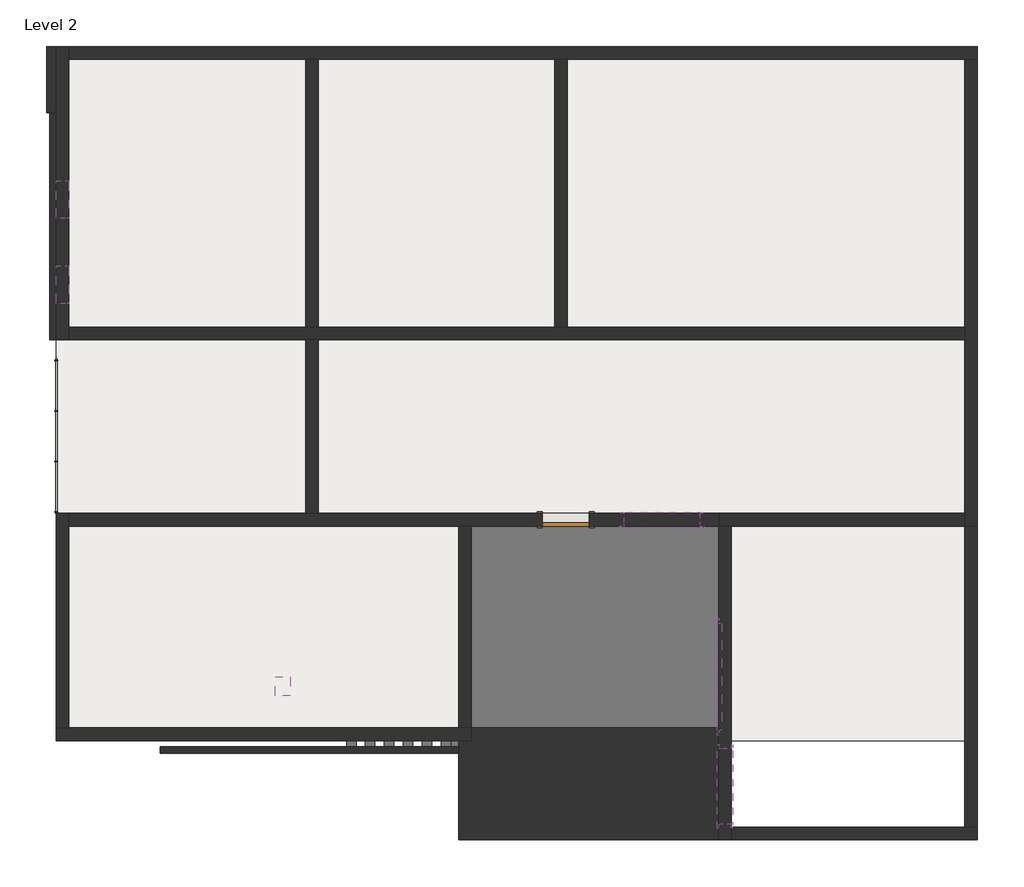
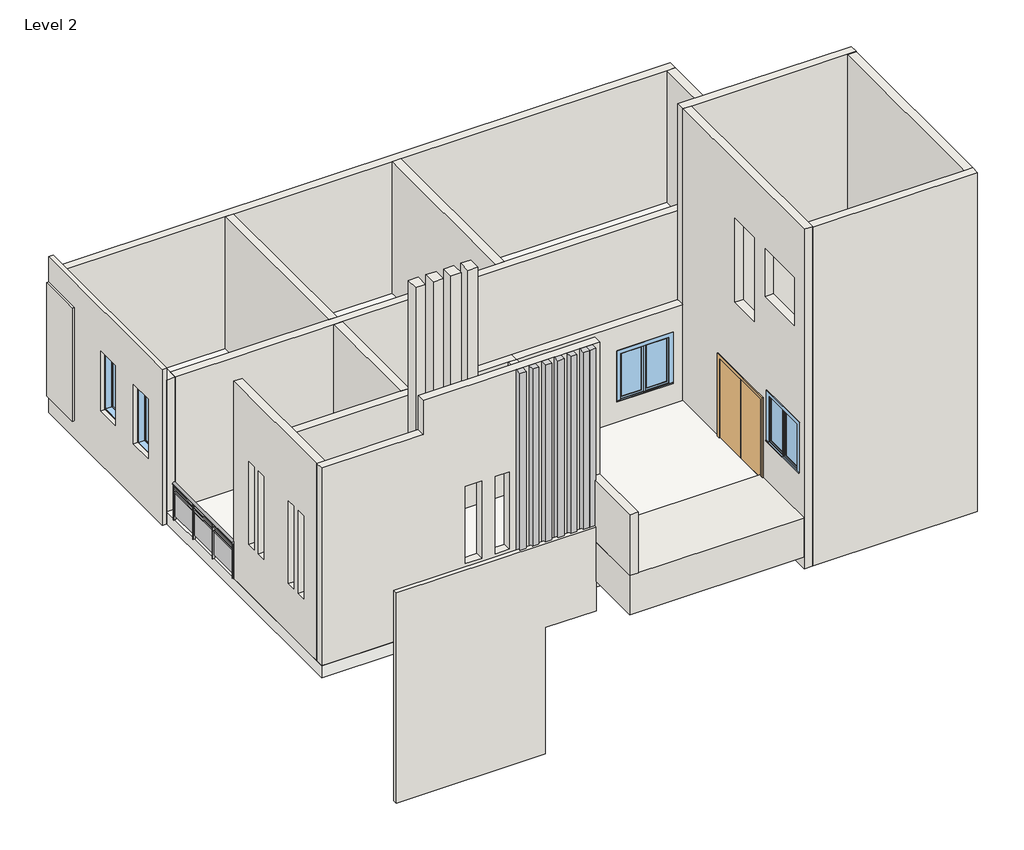
# One storey: 19 walls, 7 proxies, 4 windows, 2 doors, 2 roofs, 1 railing.
"""IFC4 building model written with IfcOpenShell, lengths in millimetres."""

from ifc_helpers import new_model, si_unit, point, frame, origin, place, context, project, spatial, polyline, ellipse_curve, trimmed, outline, extrude, faceted_brep, transform, mapped, element, save
from ifc_brep_helpers import plane_surface, extruded_surface, advanced_brep
from components import door_aae36eb6, door_b6acaa4e, walls_2_walls_1_41e9462b, walls_4_walls_4_3d1cd982, walls_6_walls_6_eb98cddc, window_0862ab64, window_8561b6b6

model = new_model("IFC4")

# Units and contexts
model_context = context("Model", 3, world=origin())
ifc_project = project(units=[si_unit("LENGTHUNIT", "METRE", prefix="MILLI")], contexts=[model_context])

# Site, building, storey
site = spatial("IfcSite", under=ifc_project)
building = spatial("IfcBuilding", under=site)
storey = spatial("IfcBuildingStorey", under=building, Name="Level 2", Elevation=3657.6)

# Proxies
placement = place(None, origin())
element("IfcBuildingElementProxy", 1, Name="Cornice", ObjectType="Cornice", at=placement, inside=storey, context=model_context, shape_type="SweptSolid", body=[
    extrude(outline(polyline([(-6382.6620963, -3412.0885822), (-6382.6620963, -3564.4885822), (-6535.0620963, -3564.4885822), (-6535.0620963, -3412.0885822), (-6382.6620963, -3412.0885822)])), frame((0.0, 0.0, 3962.4), z_axis=(0.0, 0.0, 1.0), x_axis=(1.0, 0.0, 0.0)), (0.0, 0.0, 1.0), 5885.4766226),
])
element("IfcBuildingElementProxy", 2, Name="Cornice", ObjectType="Cornice", at=placement, inside=storey, context=model_context, shape_type="SweptSolid", body=[
    extrude(outline(polyline([(-6077.8620963, -3412.0885822), (-6077.8620963, -3564.4885822), (-6230.2620963, -3564.4885822), (-6230.2620963, -3412.0885822), (-6077.8620963, -3412.0885822)])), frame((0.0, 0.0, 3962.4), z_axis=(0.0, 0.0, 1.0), x_axis=(1.0, 0.0, 0.0)), (0.0, 0.0, 1.0), 5885.4766226),
])
element("IfcBuildingElementProxy", 3, Name="Cornice", ObjectType="Cornice", at=placement, inside=storey, context=model_context, shape_type="SweptSolid", body=[
    extrude(outline(polyline([(-5773.0620963, -3412.0885822), (-5773.0620963, -3564.4885822), (-5925.4620963, -3564.4885822), (-5925.4620963, -3412.0885822), (-5773.0620963, -3412.0885822)])), frame((0.0, 0.0, 3962.4), z_axis=(0.0, 0.0, 1.0), x_axis=(1.0, 0.0, 0.0)), (0.0, 0.0, 1.0), 5885.4766226),
])
element("IfcBuildingElementProxy", 4, Name="Cornice", ObjectType="Cornice", at=placement, inside=storey, context=model_context, shape_type="SweptSolid", body=[
    extrude(outline(polyline([(-5468.2620963, -3412.0885822), (-5468.2620963, -3564.4885822), (-5620.6620963, -3564.4885822), (-5620.6620963, -3412.0885822), (-5468.2620963, -3412.0885822)])), frame((0.0, 0.0, 3962.4), z_axis=(0.0, 0.0, 1.0), x_axis=(1.0, 0.0, 0.0)), (0.0, 0.0, 1.0), 5885.4766226),
])
element("IfcBuildingElementProxy", 5, Name="Cornice", ObjectType="Cornice", at=placement, inside=storey, context=model_context, shape_type="SweptSolid", body=[
    extrude(outline(polyline([(-5163.4620963, -3412.0885822), (-5163.4620963, -3564.4885822), (-5315.8620963, -3564.4885822), (-5315.8620963, -3412.0885822), (-5163.4620963, -3412.0885822)])), frame((0.0, 0.0, 3962.4), z_axis=(0.0, 0.0, 1.0), x_axis=(1.0, 0.0, 0.0)), (0.0, 0.0, 1.0), 5885.4766226),
])
element("IfcBuildingElementProxy", 6, Name="Cornice", ObjectType="Cornice", at=placement, inside=storey, context=model_context, shape_type="SweptSolid", body=[
    extrude(outline(polyline([(-4858.6620963, -3412.0885822), (-4858.6620963, -3564.4885822), (-5011.0620963, -3564.4885822), (-5011.0620963, -3412.0885822), (-4858.6620963, -3412.0885822)])), frame((0.0, 0.0, 3962.4), z_axis=(0.0, 0.0, 1.0), x_axis=(1.0, 0.0, 0.0)), (0.0, 0.0, 1.0), 5885.4766226),
])
element("IfcBuildingElementProxy", 7, Name="Cornice", ObjectType="Cornice", at=placement, inside=storey, context=model_context, shape_type="SweptSolid", body=[
    extrude(outline(polyline([(-4706.2620963, -3412.0885822), (-4706.2620963, -3564.4885822), (-4858.6620963, -3564.4885822), (-4858.6620963, -3412.0885822), (-4706.2620963, -3412.0885822)])), frame((0.0, 0.0, 3962.4), z_axis=(0.0, 0.0, 1.0), x_axis=(1.0, 0.0, 0.0)), (0.0, 0.0, 1.0), 5885.4766226),
])

# Doors
door_shape = door_aae36eb6(model_context)
element("IfcDoor", 8, ObjectType="Door-Double-Flush_Panel : 68\" x 80\"", at=placement, inside=storey, context=model_context, shape_type="MappedRepresentation", body=[
    mapped(door_shape, transform((-439.0620963, -2383.3885822, 4876.8), x_axis=(0.0, 1.0, 0.0), y_axis=(-1.0, 0.0, 0.0), z_axis=(0.0, 0.0, 1.0))),
])
door_2_shape = door_b6acaa4e(model_context)
element("IfcDoor", 9, ObjectType="Single-Flush : 30\" x 84\"", at=placement, inside=storey, context=model_context, shape_type="MappedRepresentation", body=[
    mapped(door_2_shape, transform((-3004.4620963, 143.9114178, 4673.6), x_axis=(-1.0, 0.0, 0.0), y_axis=(0.0, -1.0, 0.0), z_axis=(0.0, 0.0, 1.0))),
])

# Railing
element("IfcRailing", 10, ObjectType="Glass Panel - Bottom Fill", at=placement, inside=storey, context=model_context, shape_type="SolidModel", body=[
    advanced_brep(
    [(-11170.5620963, 2730.1130309, 4876.8), (-11246.7620963, 2730.1130309, 4876.8), (-11170.5620963, 245.5114178, 4876.8), (-11246.7620963, 245.5114178, 4876.8)],
    [
        (0, 1, ellipse_curve(frame((-11208.6620963, 2730.1130309, 4876.8), z_axis=(0.0, 1.0, 0.0), x_axis=(-1.0, 0.0, 0.0)), 38.1, 28.575)),
        (1, 0, ellipse_curve(frame((-11208.6620963, 2730.1130309, 4876.8), z_axis=(0.0, 1.0, 0.0), x_axis=(-1.0, 0.0, 0.0)), 38.1, 28.575)),
        (2, 3, ellipse_curve(frame((-11208.6620963, 245.5114178, 4876.8), z_axis=(0.0, -1.0, 0.0), x_axis=(-1.0, 0.0, 0.0)), 38.1, 28.575)),
        (3, 2, ellipse_curve(frame((-11208.6620963, 245.5114178, 4876.8), z_axis=(0.0, -1.0, 0.0), x_axis=(-1.0, 0.0, 0.0)), 38.1, 28.575)),
        (0, 2),
        (3, 1),
    ],
    [
        plane_surface(frame((-11208.6620963, 2730.1130309, 4876.8), z_axis=(0.0, 1.0, 0.0), x_axis=(0.0, 0.0, -1.0))),
        plane_surface(frame((-11208.6620963, 245.5114178, 4876.8), z_axis=(0.0, -1.0, 0.0), x_axis=(0.0, 0.0, -1.0))),
        extruded_surface(trimmed(ellipse_curve(frame((-11208.6620963, 245.5114178, 4876.8), z_axis=(0.0, 1.0, 0.0), x_axis=(-1.0, 0.0, 0.0)), 38.1, 28.575), [point((-11170.5620963, 245.5114178, 4876.8))], [point((-11246.7620963, 245.5114178, 4876.8))], True, "CARTESIAN"), (0.0, 2484.6016131, 0.0), 2484.6016131),
        extruded_surface(trimmed(ellipse_curve(frame((-11208.6620963, 245.5114178, 4876.8), z_axis=(0.0, 1.0, 0.0), x_axis=(-1.0, 0.0, 0.0)), 38.1, 28.575), [point((-11246.7620963, 245.5114178, 4876.8))], [point((-11170.5620963, 245.5114178, 4876.8))], True, "CARTESIAN"), (0.0, 2484.6016131, 0.0), 2484.6016131),
    ],
    [
        (0, [[1, 2]]),
        (1, [[3, 4]]),
        (2, [[-1, 5, -4, 6]]),
        (3, [[-2, -6, -3, -5]]),
    ],
),
    extrude(outline(polyline([(-11221.3620963, 2730.1130309), (-11195.9620963, 2730.1130309), (-11195.9620963, 245.5114178), (-11221.3620963, 245.5114178), (-11221.3620963, 2730.1130309)])), frame((0.0, 0.0, 4762.5), z_axis=(0.0, 0.0, 1.0), x_axis=(1.0, 0.0, 0.0)), (0.0, 0.0, 1.0), 25.4),
    extrude(outline(polyline([(-11221.3620963, 2730.1130309), (-11195.9620963, 2730.1130309), (-11195.9620963, 245.5114178), (-11221.3620963, 245.5114178), (-11221.3620963, 2730.1130309)])), frame((0.0, 0.0, 4660.9), z_axis=(0.0, 0.0, 1.0), x_axis=(1.0, 0.0, 0.0)), (0.0, 0.0, 1.0), 25.4),
    extrude(outline(polyline([(-11234.0620963, 274.9622243), (-11183.2620963, 274.9622243), (-11183.2620963, 262.2622243), (-11234.0620963, 262.2622243), (-11234.0620963, 274.9622243)])), frame((0.0, 0.0, 3962.4), z_axis=(0.0, 0.0, 1.0), x_axis=(1.0, 0.0, 0.0)), (0.0, 0.0, 1.0), 885.6788223),
    extrude(outline(polyline([(-11202.1269393, 1081.4122243), (-11202.1269393, 268.6122243), (-11208.4769393, 268.6122243), (-11208.4769393, 1081.4122243), (-11202.1269393, 1081.4122243)])), frame((0.0, 0.0, 4064.0), z_axis=(0.0, 0.0, 1.0), x_axis=(1.0, 0.0, 0.0)), (0.0, 0.0, 1.0), 596.9),
    extrude(outline(polyline([(-11234.0620963, 1087.7622243), (-11183.2620963, 1087.7622243), (-11183.2620963, 1075.0622243), (-11234.0620963, 1075.0622243), (-11234.0620963, 1087.7622243)])), frame((0.0, 0.0, 3962.4), z_axis=(0.0, 0.0, 1.0), x_axis=(1.0, 0.0, 0.0)), (0.0, 0.0, 1.0), 885.6788223),
    extrude(outline(polyline([(-11202.1269393, 1894.2122243), (-11202.1269393, 1081.4122243), (-11208.4769393, 1081.4122243), (-11208.4769393, 1894.2122243), (-11202.1269393, 1894.2122243)])), frame((0.0, 0.0, 4064.0), z_axis=(0.0, 0.0, 1.0), x_axis=(1.0, 0.0, 0.0)), (0.0, 0.0, 1.0), 596.9),
    extrude(outline(polyline([(-11234.0620963, 1900.5622243), (-11183.2620963, 1900.5622243), (-11183.2620963, 1887.8622243), (-11234.0620963, 1887.8622243), (-11234.0620963, 1900.5622243)])), frame((0.0, 0.0, 3962.4), z_axis=(0.0, 0.0, 1.0), x_axis=(1.0, 0.0, 0.0)), (0.0, 0.0, 1.0), 885.6788223),
    extrude(outline(polyline([(-11202.1269393, 2707.0122243), (-11202.1269393, 1894.2122243), (-11208.4769393, 1894.2122243), (-11208.4769393, 2707.0122243), (-11202.1269393, 2707.0122243)])), frame((0.0, 0.0, 4064.0), z_axis=(0.0, 0.0, 1.0), x_axis=(1.0, 0.0, 0.0)), (0.0, 0.0, 1.0), 596.9),
    extrude(outline(polyline([(-11234.0620963, 2713.3622243), (-11183.2620963, 2713.3622243), (-11183.2620963, 2700.6622243), (-11234.0620963, 2700.6622243), (-11234.0620963, 2713.3622243)])), frame((0.0, 0.0, 3962.4), z_axis=(0.0, 0.0, 1.0), x_axis=(1.0, 0.0, 0.0)), (0.0, 0.0, 1.0), 885.6788223),
    extrude(outline(polyline([(-11218.1870963, 258.2114178), (-11199.1370963, 258.2114178), (-11199.1370963, 239.1614178), (-11218.1870963, 239.1614178), (-11218.1870963, 258.2114178)])), frame((0.0, 0.0, 3962.4), z_axis=(0.0, 0.0, 1.0), x_axis=(1.0, 0.0, 0.0)), (0.0, 0.0, 1.0), 885.6788223),
    extrude(outline(polyline([(-11218.1870963, 2736.4630309), (-11199.1370963, 2736.4630309), (-11199.1370963, 2717.4130309), (-11218.1870963, 2717.4130309), (-11218.1870963, 2736.4630309)])), frame((0.0, 0.0, 3962.4), z_axis=(0.0, 0.0, 1.0), x_axis=(1.0, 0.0, 0.0)), (0.0, 0.0, 1.0), 885.6788223),
])

# Roofs
element("IfcRoof", 11, ObjectType="Generic - 12\"", at=placement, inside=storey, context=model_context, shape_type="SweptSolid", body=[
    extrude(outline(polyline([(-11208.6620963, 7763.9114178), (3624.9379037, 7763.9114178), (3624.9379037, -3412.0885822), (-11208.6620963, -3412.0885822), (-11208.6620963, 7763.9114178)])), frame((0.0, 0.0, 3657.6), z_axis=(0.0, 0.0, 1.0), x_axis=(1.0, 0.0, 0.0)), (0.0, 0.0, 1.0), 304.8),
])
element("IfcRoof", 12, ObjectType="Generic - 12\"", at=placement, inside=storey, context=model_context, shape_type="SweptSolid", body=[
    extrude(outline(polyline([(-4528.4620963, 42.3114178), (-540.6620963, 42.3114178), (-540.6620963, -3208.8885822), (-4528.4620963, -3208.8885822), (-4528.4620963, 42.3114178)])), frame((0.0, 0.0, 4572.0), z_axis=(0.0, 0.0, 1.0), x_axis=(1.0, 0.0, 0.0)), (0.0, 0.0, 1.0), 304.8),
])

# Walls
element("IfcWall", 13, ObjectType="Generic - 4\" Brick", at=placement, inside=storey, context=model_context, shape_type="SweptSolid", body=[
    extrude(outline(polyline([(0.0, -9532.2620963), (0.0, -5950.8620963), (3214.2753526, -5950.8620963), (3214.2753526, -4731.6620963), (5347.8753526, -4731.6620963), (5347.8753526, -9532.2620963), (0.0, -9532.2620963)])), frame((0.0, -3615.2885822, 0.0), z_axis=(0.0, 1.0, 0.0), x_axis=(0.0, 0.0, 1.0)), (0.0, 0.0, 1.0), 101.6),
])
element("IfcWall", 14, ObjectType="Generic - 8\"", at=placement, inside=storey, context=model_context, shape_type="Brep", body=[
    faceted_brep([(-11005.4620963, 42.3114178, 3657.6), (-4731.6620963, 42.3114178, 3657.6), (-4528.4620963, 42.3114178, 3657.6), (-540.6620963, 42.3114178, 3657.6), (-540.6620963, 42.3114178, 7315.2), (-4496.7120963, 42.3114178, 7315.2), (-4528.4620963, 42.3114178, 7315.2), (-4731.6620963, 42.3114178, 7315.2), (-11005.4620963, 42.3114178, 7315.2), (-2623.4620963, 42.3114178, 4673.6), (-3385.4620963, 42.3114178, 4673.6), (-3385.4620963, 42.3114178, 6807.2), (-2623.4620963, 42.3114178, 6807.2), (-2064.6620963, 42.3114178, 6627.1844353), (-845.4620963, 42.3114178, 6627.1844353), (-845.4620963, 42.3114178, 5407.9844353), (-2064.6620963, 42.3114178, 5407.9844353), (-11005.4620963, 245.5114178, 3657.6), (-11005.4620963, 245.5114178, 3962.4), (-11005.4620963, 245.5114178, 7315.2), (-7195.4620963, 245.5114178, 7315.2), (-6992.2620963, 245.5114178, 7315.2), (-4528.4620963, 245.5114178, 7315.2), (-4496.7120963, 245.5114178, 7315.2), (-540.6620963, 245.5114178, 7315.2), (-540.6620963, 245.5114178, 3657.6), (-6992.2620963, 245.5114178, 3657.6), (-7195.4620963, 245.5114178, 3657.6), (-2623.4620963, 245.5114178, 4673.6), (-2623.4620963, 245.5114178, 6807.2), (-3385.4620963, 245.5114178, 6807.2), (-3385.4620963, 245.5114178, 4673.6), (-2064.6620963, 245.5114178, 6627.1844353), (-2064.6620963, 245.5114178, 5407.9844353), (-845.4620963, 245.5114178, 5407.9844353), (-845.4620963, 245.5114178, 6627.1844353)], [[[0, 1, 2, 3, 4, 5, 6, 7, 8], [9, 10, 11, 12], [13, 14, 15, 16]], [[17, 18, 19, 20, 21, 22, 23, 24, 25, 26, 27], [28, 29, 30, 31], [32, 33, 34, 35]], [[3, 2, 1, 0, 17, 27, 26, 25]], [[4, 3, 25, 24]], [[6, 5, 4, 24, 23, 22]], [[0, 8, 19, 18, 17]], [[8, 7, 6, 22, 21, 20, 19]], [[10, 9, 28, 31]], [[11, 10, 31, 30]], [[12, 11, 30, 29]], [[9, 12, 29, 28]], [[33, 32, 13, 16]], [[34, 33, 16, 15]], [[35, 34, 15, 14]], [[32, 35, 14, 13]]]),
])
element("IfcWall", 15, ObjectType="Generic - 8\"", at=placement, inside=storey, context=model_context, shape_type="Brep", body=[
    faceted_brep([(-11005.4620963, 3039.5114178, 3657.6), (-11005.4620963, 3242.7114178, 3657.6), (-11005.4620963, 7560.7114178, 3657.6), (-11005.4620963, 7763.9114178, 3657.6), (-11005.4620963, 7763.9114178, 7315.2), (-11005.4620963, 7560.7114178, 7315.2), (-11005.4620963, 3242.7114178, 7315.2), (-11005.4620963, 3039.5114178, 7315.2), (-11005.4620963, 3623.7114178, 6513.5923365), (-11005.4620963, 4233.3114178, 6513.5923365), (-11005.4620963, 4233.3114178, 4989.5923365), (-11005.4620963, 3623.7114178, 4989.5923365), (-11005.4620963, 4995.3114178, 6537.7138354), (-11005.4620963, 5604.9114178, 6537.7138354), (-11005.4620963, 5604.9114178, 5013.7138354), (-11005.4620963, 4995.3114178, 5013.7138354), (-11208.6620963, 3039.5114178, 3657.6), (-11208.6620963, 3039.5114178, 7315.2), (-11208.6620963, 7763.9114178, 7315.2), (-11208.6620963, 7763.9114178, 3657.6), (-11208.6620963, 3623.7114178, 6513.5923365), (-11208.6620963, 3623.7114178, 4989.5923365), (-11208.6620963, 4233.3114178, 4989.5923365), (-11208.6620963, 4233.3114178, 6513.5923365), (-11208.6620963, 4995.3114178, 6537.7138354), (-11208.6620963, 4995.3114178, 5013.7138354), (-11208.6620963, 5604.9114178, 5013.7138354), (-11208.6620963, 5604.9114178, 6537.7138354)], [[[0, 1, 2, 3, 4, 5, 6, 7], [8, 9, 10, 11], [12, 13, 14, 15]], [[16, 17, 18, 19], [20, 21, 22, 23], [24, 25, 26, 27]], [[3, 2, 1, 0, 16, 19]], [[4, 3, 19, 18]], [[0, 7, 17, 16]], [[7, 6, 5, 4, 18, 17]], [[21, 20, 8, 11]], [[22, 21, 11, 10]], [[23, 22, 10, 9]], [[20, 23, 9, 8]], [[25, 24, 12, 15]], [[26, 25, 15, 14]], [[27, 26, 14, 13]], [[24, 27, 13, 12]]]),
])
element("IfcWall", 16, ObjectType="Generic - 8\"", at=placement, inside=storey, context=model_context, shape_type="Brep", body=[
    faceted_brep([(-11005.4620963, 7560.7114178, 3657.6), (-7195.4620963, 7560.7114178, 3657.6), (-6992.2620963, 7560.7114178, 3657.6), (-3182.2620963, 7560.7114178, 3657.6), (-2979.0620963, 7560.7114178, 3657.6), (3421.7379037, 7560.7114178, 3657.6), (3624.9379037, 7560.7114178, 3657.6), (3624.9379037, 7560.7114178, 7315.2), (3421.7379037, 7560.7114178, 7315.2), (-2979.0620963, 7560.7114178, 7315.2), (-3182.2620963, 7560.7114178, 7315.2), (-6992.2620963, 7560.7114178, 7315.2), (-7195.4620963, 7560.7114178, 7315.2), (-11005.4620963, 7560.7114178, 7315.2), (-11005.4620963, 7763.9114178, 3657.6), (-11005.4620963, 7763.9114178, 7315.2), (3624.9379037, 7763.9114178, 7315.2), (3624.9379037, 7763.9114178, 3657.6)], [[[0, 1, 2, 3, 4, 5, 6, 7, 8, 9, 10, 11, 12, 13]], [[14, 15, 16, 17]], [[6, 5, 4, 3, 2, 1, 0, 14, 17]], [[0, 13, 15, 14]], [[7, 6, 17, 16]], [[13, 12, 11, 10, 9, 8, 7, 16, 15]]]),
])
element("IfcWall", 17, ObjectType="Generic - 8\"", at=placement, inside=storey, context=model_context, shape_type="Brep", body=[
    faceted_brep([(3421.7379037, 7560.7114178, 3657.6), (3421.7379037, 3242.7114178, 3657.6), (3421.7379037, 3039.5114178, 3657.6), (3421.7379037, 245.5114178, 3657.6), (3421.7379037, 42.3114178, 3657.6), (3421.7379037, 42.3114178, 7315.2), (3421.7379037, 245.5114178, 7315.2), (3421.7379037, 3039.5114178, 7315.2), (3421.7379037, 3242.7114178, 7315.2), (3421.7379037, 7560.7114178, 7315.2), (3624.9379037, 7560.7114178, 3657.6), (3624.9379037, 7560.7114178, 7315.2), (3624.9379037, 245.5114178, 7315.2), (3624.9379037, 42.3114178, 7315.2), (3624.9379037, 42.3114178, 3657.6)], [[[0, 1, 2, 3, 4, 5, 6, 7, 8, 9]], [[10, 11, 12, 13, 14]], [[4, 3, 2, 1, 0, 10, 14]], [[0, 9, 11, 10]], [[5, 4, 14, 13]], [[6, 5, 13, 12]], [[9, 8, 7, 6, 12, 11]]]),
])
element("IfcWall", 18, ObjectType="Generic - 8\"", at=placement, inside=storey, context=model_context, shape_type="Brep", body=[
    faceted_brep([(3421.7379037, 245.5114178, 3657.6), (-540.6620963, 245.5114178, 3657.6), (-540.6620963, 245.5114178, 7315.2), (-540.6620963, 245.5114178, 12289.4988159), (3624.9379037, 245.5114178, 12289.4988159), (3624.9379037, 245.5114178, 10972.8), (3624.9379037, 245.5114178, 7315.2), (3421.7379037, 245.5114178, 7315.2), (3421.7379037, 42.3114178, 3657.6), (3421.7379037, 42.3114178, 7315.2), (3624.9379037, 42.3114178, 7315.2), (3624.9379037, 42.3114178, 12274.5893011), (3624.9379037, 42.3114178, 12289.4988159), (-337.4620963, 42.3114178, 12289.4988159), (-540.6620963, 42.3114178, 12289.4988159), (-540.6620963, 42.3114178, 7315.2), (-540.6620963, 42.3114178, 3657.6), (-337.4620963, 42.3114178, 3657.6)], [[[0, 1, 2, 3, 4, 5, 6, 7]], [[8, 9, 10, 11, 12, 13, 14, 15, 16, 17]], [[1, 0, 8, 17, 16]], [[4, 3, 14, 13, 12]], [[1, 16, 15, 14, 3, 2]], [[6, 10, 9, 7]], [[0, 7, 9, 8]], [[4, 12, 11, 10, 6, 5]]]),
])
element("IfcWall", 19, ObjectType="Generic - 8\"", at=placement, inside=storey, context=model_context, shape_type="Brep", body=[
    faceted_brep([(-540.6620963, 42.3114178, 3657.6), (-540.6620963, -5012.2885822, 3657.6), (-540.6620963, -5012.2885822, 12289.4988159), (-540.6620963, 42.3114178, 12289.4988159), (-540.6620963, -1519.7885822, 4876.8), (-540.6620963, -1519.7885822, 6908.8), (-540.6620963, -3246.9885822, 6908.8), (-540.6620963, -3246.9885822, 4876.8), (-540.6620963, -2942.1885822, 8686.8), (-540.6620963, -2129.3885822, 8686.8), (-540.6620963, -2129.3885822, 10820.4), (-540.6620963, -2942.1885822, 10820.4), (-540.6620963, -3386.6885822, 9594.9318944), (-540.6620963, -3386.6885822, 10814.1318944), (-540.6620963, -4605.8885822, 10814.1318944), (-540.6620963, -4605.8885822, 9594.9318944), (-540.6620963, -3539.0885822, 5985.020216), (-540.6620963, -3539.0885822, 7204.220216), (-540.6620963, -4758.2885822, 7204.220216), (-540.6620963, -4758.2885822, 5985.020216), (-337.4620963, -5012.2885822, 3657.6), (-337.4620963, -4809.0885822, 3657.6), (-337.4620963, 42.3114178, 3657.6), (-337.4620963, 42.3114178, 12289.4988159), (-337.4620963, -5012.2885822, 12289.4988159), (-337.4620963, -5012.2885822, 12274.5893011), (-337.4620963, -1519.7885822, 6908.8), (-337.4620963, -1519.7885822, 4876.8), (-337.4620963, -3246.9885822, 4876.8), (-337.4620963, -3246.9885822, 6908.8), (-337.4620963, -2129.3885822, 8686.8), (-337.4620963, -2942.1885822, 8686.8), (-337.4620963, -2942.1885822, 10820.4), (-337.4620963, -2129.3885822, 10820.4), (-337.4620963, -3386.6885822, 10814.1318944), (-337.4620963, -3386.6885822, 9594.9318944), (-337.4620963, -4605.8885822, 9594.9318944), (-337.4620963, -4605.8885822, 10814.1318944), (-337.4620963, -3539.0885822, 7204.220216), (-337.4620963, -3539.0885822, 5985.020216), (-337.4620963, -4758.2885822, 5985.020216), (-337.4620963, -4758.2885822, 7204.220216)], [[[0, 1, 2, 3], [4, 5, 6, 7], [8, 9, 10, 11], [12, 13, 14, 15], [16, 17, 18, 19]], [[20, 21, 22, 23, 24, 25], [26, 27, 28, 29], [30, 31, 32, 33], [34, 35, 36, 37], [38, 39, 40, 41]], [[1, 0, 22, 21, 20]], [[3, 2, 24, 23]], [[0, 3, 23, 22]], [[2, 1, 20, 25, 24]], [[4, 27, 26, 5]], [[5, 26, 29, 6]], [[6, 29, 28, 7]], [[27, 4, 7, 28]], [[9, 8, 31, 30]], [[10, 9, 30, 33]], [[11, 10, 33, 32]], [[8, 11, 32, 31]], [[35, 34, 13, 12]], [[36, 35, 12, 15]], [[37, 36, 15, 14]], [[34, 37, 14, 13]], [[39, 38, 17, 16]], [[40, 39, 16, 19]], [[41, 40, 19, 18]], [[38, 41, 18, 17]]]),
])
element("IfcWall", 20, ObjectType="Generic - 8\"", at=placement, inside=storey, context=model_context, shape_type="Brep", body=[
    faceted_brep([(-337.4620963, -5012.2885822, 3657.6), (3624.9379037, -5012.2885822, 3657.6), (3624.9379037, -5012.2885822, 12274.5893011), (-337.4620963, -5012.2885822, 12274.5893011), (-337.4620963, -4809.0885822, 3657.6), (-337.4620963, -4809.0885822, 12274.5893011), (3421.7379037, -4809.0885822, 12274.5893011), (3624.9379037, -4809.0885822, 12274.5893011), (3624.9379037, -4809.0885822, 3657.6), (3421.7379037, -4809.0885822, 3657.6)], [[[0, 1, 2, 3]], [[4, 5, 6, 7, 8, 9]], [[1, 0, 4, 9, 8]], [[3, 2, 7, 6, 5]], [[0, 3, 5, 4]], [[2, 1, 8, 7]]]),
])
element("IfcWall", 21, ObjectType="Generic - 8\"", at=placement, inside=storey, context=model_context, shape_type="Brep", body=[
    faceted_brep([(3624.9379037, -4809.0885822, 3657.6), (3624.9379037, 42.3114178, 3657.6), (3624.9379037, 42.3114178, 7315.2), (3624.9379037, 42.3114178, 12274.5893011), (3624.9379037, -4809.0885822, 12274.5893011), (3421.7379037, -4809.0885822, 3657.6), (3421.7379037, -4809.0885822, 12274.5893011), (3421.7379037, 42.3114178, 12274.5893011), (3421.7379037, 42.3114178, 7315.2), (3421.7379037, 42.3114178, 3657.6)], [[[0, 1, 2, 3, 4]], [[5, 6, 7, 8, 9]], [[1, 0, 5, 9]], [[4, 3, 7, 6]], [[0, 4, 6, 5]], [[1, 9, 8, 7, 3, 2]]]),
])
element("IfcWall", 22, ObjectType="Generic - 8\"", at=placement, inside=storey, context=model_context, shape_type="Brep", body=[
    faceted_brep([(-11005.4620963, 3039.5114178, 3657.6), (-7195.4620963, 3039.5114178, 3657.6), (-6992.2620963, 3039.5114178, 3657.6), (3421.7379037, 3039.5114178, 3657.6), (3421.7379037, 3039.5114178, 7315.2), (-6992.2620963, 3039.5114178, 7315.2), (-7195.4620963, 3039.5114178, 7315.2), (-11005.4620963, 3039.5114178, 7315.2), (-11005.4620963, 3242.7114178, 3657.6), (-11005.4620963, 3242.7114178, 7315.2), (-7195.4620963, 3242.7114178, 7315.2), (-6992.2620963, 3242.7114178, 7315.2), (-3182.2620963, 3242.7114178, 7315.2), (-2979.0620963, 3242.7114178, 7315.2), (3421.7379037, 3242.7114178, 7315.2), (3421.7379037, 3242.7114178, 3657.6), (-2979.0620963, 3242.7114178, 3657.6), (-3182.2620963, 3242.7114178, 3657.6), (-6992.2620963, 3242.7114178, 3657.6), (-7195.4620963, 3242.7114178, 3657.6)], [[[0, 1, 2, 3, 4, 5, 6, 7]], [[8, 9, 10, 11, 12, 13, 14, 15, 16, 17, 18, 19]], [[3, 2, 1, 0, 8, 19, 18, 17, 16, 15]], [[0, 7, 9, 8]], [[4, 3, 15, 14]], [[7, 6, 5, 4, 14, 13, 12, 11, 10, 9]]]),
])
element("IfcWall", 23, ObjectType="Generic - 8\"", at=placement, inside=storey, context=model_context, shape_type="SweptSolid", body=[
    extrude(outline(polyline([(-7195.4620963, 245.5114178), (-7195.4620963, 3039.5114178), (-6992.2620963, 3039.5114178), (-6992.2620963, 245.5114178), (-7195.4620963, 245.5114178)])), frame((0.0, 0.0, 3657.6), z_axis=(0.0, 0.0, 1.0), x_axis=(1.0, 0.0, 0.0)), (0.0, 0.0, 1.0), 3657.6),
])
element("IfcWall", 24, ObjectType="Generic - 8\"", at=placement, inside=storey, context=model_context, shape_type="SweptSolid", body=[
    extrude(outline(polyline([(-2979.0620963, 7560.7114178), (-2979.0620963, 3242.7114178), (-3182.2620963, 3242.7114178), (-3182.2620963, 7560.7114178), (-2979.0620963, 7560.7114178)])), frame((0.0, 0.0, 3657.6), z_axis=(0.0, 0.0, 1.0), x_axis=(1.0, 0.0, 0.0)), (0.0, 0.0, 1.0), 3657.6),
])
element("IfcWall", 25, ObjectType="Generic - 8\"", at=placement, inside=storey, context=model_context, shape_type="SweptSolid", body=[
    extrude(outline(polyline([(-6992.2620963, 7560.7114178), (-6992.2620963, 3242.7114178), (-7195.4620963, 3242.7114178), (-7195.4620963, 7560.7114178), (-6992.2620963, 7560.7114178)])), frame((0.0, 0.0, 3657.6), z_axis=(0.0, 0.0, 1.0), x_axis=(1.0, 0.0, 0.0)), (0.0, 0.0, 1.0), 3657.6),
])
element("IfcWall", 26, ObjectType="Generic - 8\"", at=placement, inside=storey, context=model_context, shape_type="Brep", body=[
    faceted_brep([(-11208.6620963, -3412.0885822, 3962.4), (-4528.4620963, -3412.0885822, 3962.4), (-4528.4620963, -3412.0885822, 9847.8766226), (-8770.2620963, -3412.0885822, 9847.8766226), (-8770.2620963, -3412.0885822, 8984.2766226), (-11208.6620963, -3412.0885822, 8984.2766226), (-7043.0620963, -3412.0885822, 7315.2), (-6703.4763944, -3412.0885822, 7315.2), (-6703.4763944, -3412.0885822, 5347.8753526), (-7043.0620963, -3412.0885822, 5347.8753526), (-7754.2620963, -3412.0885822, 7315.2), (-7360.6785237, -3412.0885822, 7315.2), (-7360.6785237, -3412.0885822, 5347.8753526), (-7754.2620963, -3412.0885822, 5347.8753526), (-11208.6620963, -3208.8885822, 3962.4), (-11208.6620963, -3208.8885822, 8977.6089989), (-11208.6620963, -3208.8885822, 8984.2766226), (-8770.2620963, -3208.8885822, 8984.2766226), (-8770.2620963, -3208.8885822, 9847.8766226), (-4528.4620963, -3208.8885822, 9847.8766226), (-4528.4620963, -3208.8885822, 7315.2), (-4528.4620963, -3208.8885822, 3962.4), (-11005.4620963, -3208.8885822, 3962.4), (-7043.0620963, -3208.8885822, 7315.2), (-7043.0620963, -3208.8885822, 5347.8753526), (-6703.4763944, -3208.8885822, 5347.8753526), (-6703.4763944, -3208.8885822, 7315.2), (-7754.2620963, -3208.8885822, 7315.2), (-7754.2620963, -3208.8885822, 5347.8753526), (-7360.6785237, -3208.8885822, 5347.8753526), (-7360.6785237, -3208.8885822, 7315.2)], [[[0, 1, 2, 3, 4, 5], [6, 7, 8, 9], [10, 11, 12, 13]], [[14, 15, 16, 17, 18, 19, 20, 21, 22], [23, 24, 25, 26], [27, 28, 29, 30]], [[0, 5, 16, 15, 14]], [[2, 1, 21, 20, 19]], [[1, 0, 14, 22, 21]], [[3, 2, 19, 18]], [[4, 3, 18, 17]], [[5, 4, 17, 16]], [[7, 6, 23, 26]], [[8, 7, 26, 25]], [[9, 8, 25, 24]], [[6, 9, 24, 23]], [[11, 10, 27, 30]], [[12, 11, 30, 29]], [[13, 12, 29, 28]], [[10, 13, 28, 27]]]),
])
element("IfcWall", 27, ObjectType="Generic - 8\"", at=placement, inside=storey, context=model_context, shape_type="Brep", body=[
    faceted_brep([(-11208.6620963, 245.5114178, 8977.6089989), (-11208.6620963, 245.5114178, 3962.4), (-11208.6620963, -3208.8885822, 3962.4), (-11208.6620963, -3208.8885822, 8977.6089989), (-11208.6620963, -2660.4465553, 7315.2), (-11208.6620963, -2660.4465553, 5207.0), (-11208.6620963, -2431.8465553, 5207.0), (-11208.6620963, -2431.8465553, 7315.2), (-11208.6620963, -2254.0465553, 7315.2), (-11208.6620963, -2254.0465553, 5207.0), (-11208.6620963, -2025.4465553, 5207.0), (-11208.6620963, -2025.4465553, 7315.2), (-11208.6620963, -1009.4465553, 7315.2), (-11208.6620963, -1009.4465553, 5207.0), (-11208.6620963, -780.8465553, 5207.0), (-11208.6620963, -780.8465553, 7315.2), (-11208.6620963, -603.0465553, 7315.2), (-11208.6620963, -603.0465553, 5207.0), (-11208.6620963, -374.4465553, 5207.0), (-11208.6620963, -374.4465553, 7315.2), (-11005.4620963, 245.5114178, 3962.4), (-11005.4620963, 245.5114178, 7315.2), (-11005.4620963, 245.5114178, 8977.6089989), (-11005.4620963, -3208.8885822, 8977.6089989), (-11005.4620963, -3208.8885822, 3962.4), (-11005.4620963, -2660.4465553, 7315.2), (-11005.4620963, -2431.8465553, 7315.2), (-11005.4620963, -2431.8465553, 5207.0), (-11005.4620963, -2660.4465553, 5207.0), (-11005.4620963, -2254.0465553, 7315.2), (-11005.4620963, -2025.4465553, 7315.2), (-11005.4620963, -2025.4465553, 5207.0), (-11005.4620963, -2254.0465553, 5207.0), (-11005.4620963, -1009.4465553, 7315.2), (-11005.4620963, -780.8465553, 7315.2), (-11005.4620963, -780.8465553, 5207.0), (-11005.4620963, -1009.4465553, 5207.0), (-11005.4620963, -603.0465553, 7315.2), (-11005.4620963, -374.4465553, 7315.2), (-11005.4620963, -374.4465553, 5207.0), (-11005.4620963, -603.0465553, 5207.0)], [[[0, 1, 2, 3], [4, 5, 6, 7], [8, 9, 10, 11], [12, 13, 14, 15], [16, 17, 18, 19]], [[20, 21, 22, 23, 24], [25, 26, 27, 28], [29, 30, 31, 32], [33, 34, 35, 36], [37, 38, 39, 40]], [[3, 2, 24, 23]], [[0, 22, 21, 20, 1]], [[2, 1, 20, 24]], [[0, 3, 23, 22]], [[5, 4, 25, 28]], [[6, 5, 28, 27]], [[7, 6, 27, 26]], [[4, 7, 26, 25]], [[9, 8, 29, 32]], [[10, 9, 32, 31]], [[11, 10, 31, 30]], [[8, 11, 30, 29]], [[13, 12, 33, 36]], [[14, 13, 36, 35]], [[15, 14, 35, 34]], [[12, 15, 34, 33]], [[17, 16, 37, 40]], [[18, 17, 40, 39]], [[19, 18, 39, 38]], [[16, 19, 38, 37]]]),
])
element("IfcWall", 28, ObjectType="Generic - 8\"", at=placement, inside=storey, context=model_context, shape_type="Brep", body=[
    faceted_brep([(-4528.4620963, -3208.8885822, 3657.6), (-4528.4620963, 42.3114178, 3657.6), (-4528.4620963, 42.3114178, 7315.2), (-4528.4620963, -3208.8885822, 7315.2), (-4528.4620963, -3208.8885822, 3962.4), (-4731.6620963, -3208.8885822, 3657.6), (-4731.6620963, -3208.8885822, 7315.2), (-4731.6620963, 42.3114178, 7315.2), (-4731.6620963, 42.3114178, 3657.6)], [[[0, 1, 2, 3, 4]], [[5, 6, 7, 8]], [[1, 0, 5, 8]], [[3, 2, 7, 6]], [[0, 4, 3, 6, 5]], [[2, 1, 8, 7]]]),
])
walls_2_walls_1_shape = walls_2_walls_1_41e9462b(model_context)
element("IfcWall", 29, ObjectType="Walls 2 : Walls 1", at=placement, inside=storey, context=model_context, shape_type="MappedRepresentation", body=[
    mapped(walls_2_walls_1_shape, transform((0.0, 0.0, 0.0), x_axis=(1.0, 0.0, 0.0), y_axis=(0.0, 1.0, 0.0), z_axis=(0.0, 0.0, 1.0))),
])
walls_4_walls_4_shape = walls_4_walls_4_3d1cd982(model_context)
element("IfcWall", 30, ObjectType="Walls 4 : Walls 4", at=placement, inside=storey, context=model_context, shape_type="MappedRepresentation", body=[
    mapped(walls_4_walls_4_shape, transform((0.0, 0.0, 0.0), x_axis=(1.0, 0.0, 0.0), y_axis=(0.0, 1.0, 0.0), z_axis=(0.0, 0.0, 1.0))),
])
walls_6_walls_6_shape = walls_6_walls_6_eb98cddc(model_context)
element("IfcWall", 31, ObjectType="Walls 6 : Walls 6", at=placement, inside=storey, context=model_context, shape_type="MappedRepresentation", body=[
    mapped(walls_6_walls_6_shape, transform((0.0, 0.0, 0.0), x_axis=(1.0, 0.0, 0.0), y_axis=(0.0, 1.0, 0.0), z_axis=(0.0, 0.0, 1.0))),
])

# Windows
window_shape = window_0862ab64(model_context)
element("IfcWindow", 32, ObjectType="Casement Dbl with Trim.0001 : 48\" x 48\"", at=placement, inside=storey, context=model_context, shape_type="MappedRepresentation", body=[
    mapped(window_shape, transform((-420.0120963, -4148.6885822, 5070.620216), x_axis=(0.0, 1.0, 0.0), y_axis=(-1.0, 0.0, 0.0), z_axis=(0.0, 0.0, 1.0))),
])
element("IfcWindow", 33, ObjectType="Casement Dbl with Trim.0001 : 48\" x 48\"", at=placement, inside=storey, context=model_context, shape_type="MappedRepresentation", body=[
    mapped(window_shape, transform((-1455.0620963, 162.9614178, 4493.5844353), x_axis=(-1.0, 0.0, 0.0), y_axis=(0.0, -1.0, 0.0), z_axis=(0.0, 0.0, 1.0))),
])
window_2_shape = window_8561b6b6(model_context)
element("IfcWindow", 34, ObjectType="Fixed : 24\" x 60\"", at=placement, inside=storey, context=model_context, shape_type="MappedRepresentation", body=[
    mapped(window_2_shape, transform((-11107.0620963, 3890.4114178, 4075.1923365), x_axis=(0.0, -1.0, 0.0), y_axis=(1.0, 0.0, 0.0), z_axis=(0.0, 0.0, 1.0))),
])
element("IfcWindow", 35, ObjectType="Fixed : 24\" x 60\"", at=placement, inside=storey, context=model_context, shape_type="MappedRepresentation", body=[
    mapped(window_2_shape, transform((-11107.0620963, 5262.0114178, 4099.3138354), x_axis=(0.0, -1.0, 0.0), y_axis=(1.0, 0.0, 0.0), z_axis=(0.0, 0.0, 1.0))),
])

save(model, "model.ifc")

# Revit data of these elements
# Type "Door-Double-Flush_Panel : 68\" x 80\""
#   Type Mark = "8"
#   Construction Type Id = "DOOR"
#   Assembly Code = "C1020"
#   Analytic Construction = "Wooden"
#   Thickness = 0' - 2"
#   Thermal Resistance (R) = 2.5876 (h·ft²·°F)/BTU
#   Swing Angle [instance default] = 90.00°
#   Panel Width = 2' - 10"
#   Heat Transfer Coefficient (U) = 0.3865 BTU/(h·ft²·°F)
#   Height = 6' - 8"
#   Trim Projection Ext = 0' - 1"
#   Trim Projection Int = 0' - 1"
#   Trim Width = 0' - 3"
#   Width = 5' - 8"
#   Define Thermal Properties by = 1
#   Panel Material = Wood - Birch - Solid Stained Light Low Gloss
#   Trim Material = Paint - Sienna
#   Visual Light Transmittance = 0
#   Solar Heat Gain Coefficient = 0
#   Function = (empty or 0)
#   Wall Closure = (empty or 0)
# Type "Single-Flush : 30\" x 84\""
#   Type Mark = "4"
#   Construction Type Id = "MDOOR"
#   Assembly Code = "C1020"
#   Analytic Construction = "Metal"
#   Thickness = 0' - 2"
#   Heat Transfer Coefficient (U) = 0.651978 BTU/(h·ft²·°F)
#   Height = 7' - 0"
#   Trim Projection Ext = 0' - 1"
#   Trim Projection Int = 0' - 1"
#   Trim Width = 0' - 3"
#   Width = 2' - 6"
#   Define Thermal Properties by = 1
#   Door Material = Door - Panel
#   Frame Material = Door - Frame
#   Visual Light Transmittance = 0
#   Solar Heat Gain Coefficient = 0
#   Function = (empty or 0)
#   Wall Closure = (empty or 0)
# Type "Glass Panel - Bottom Fill"
#   Assembly Code = "C2010400"
#   built-in parameter 1008612 = 0.0416667 (stored number, unit not read)
#   built-in parameter 1008611 = 0.0416667 (stored number, unit not read)
#   built-in parameter 1008609 = 0.333333 (stored number, unit not read)
#   built-in parameter 1008604 = 0.166667 (stored number, unit not read)
#   built-in parameter 1008603 = 0.166667 (stored number, unit not read)
#   Railing Height = 3' - 0"
#   built-in parameter 1008630 = 2
#   built-in parameter 1008610 = 2
#   built-in parameter 1008618 = Baluster - Square : 3/4"
# Type "Generic - 12\""
#   Assembly Code = "B1020"
#   Layers, outside or top first: 1' - 0" no material (function 1)
# Type "Generic - 4\" Brick"
#   Assembly Code = "B2010"
#   Layers, outside or top first: 0' - 4" "Brick, Common" (function 1)
# Type "Generic - 8\""
#   Assembly Code = "B2010"
#   Layers, outside or top first: 0' - 8" no material (function 1)
# Type "Casement Dbl with Trim.0001 : 48\" x 48\""
#   Type Mark = "10"
#   Construction Type Id = "GSP4R"
#   Assembly Code = "B2020100"
#   Analytic Construction = "1/8 in Pilkington single glazing"
#   Visual Light Transmittance = 0.9
#   Solar Heat Gain Coefficient = 0.78
#   Heat Transfer Coefficient (U) = 0.6496 BTU/(h·ft²·°F)
#   Height = 4' - 0"
#   Default Sill Height = 3' - 0"
#   Trim Projection - Ext. = 0' - 0 1/2"
#   Trim Projection - Int. = 0' - 0 3/4"
#   Trim Width - Exterior = 0' - 3 1/2"
#   Trim Width - Interior = 0' - 3 1/2"
#   Width = 4' - 0"
#   Window Inset = 0' - 0 3/4"
#   Define Thermal Properties by = 1
#   Glass Pane Material = Glass
#   Sash Material = Sash
#   Trim Exterior Material = Trim
#   Trim Interior Material = Trim
#   Wall Closure = (empty or 0)
# Type "Fixed : 24\" x 60\""
#   Type Mark = "5"
#   Construction Type Id = "GSP4R"
#   Assembly Code = "B2020100"
#   Analytic Construction = "1/8 in Pilkington single glazing"
#   Visual Light Transmittance = 0.9
#   Solar Heat Gain Coefficient = 0.78
#   Heat Transfer Coefficient (U) = 0.6496 BTU/(h·ft²·°F)
#   Height = 5' - 0"
#   Default Sill Height = 3' - 0"
#   Width = 2' - 0"
#   Window Inset = 0' - 0 3/4"
#   Define Thermal Properties by = 1
#   Glass Pane Material = Glass
#   Sash Material = Sash
#   Wall Closure = (empty or 0)
# Elements 1, 2, 3, 4, 5, 6, 7 (IfcBuildingElementProxy, "Cornice")
#   Phase Created = New Construction
#   Materials on its faces: "Default Wall"
# Element 8 (IfcDoor, "Door-Double-Flush_Panel : 68\" x 80\"")
#   Swing Angle = 90.00°
#   Phase Created = New Construction
#   Materials on its faces: "Paint - Sienna", "Wood - Birch - Solid Stained Light Low Gloss"
# Element 9 (IfcDoor, "Single-Flush : 30\" x 84\"")
#   Phase Created = New Construction
#   Materials on its faces: "Door - Frame", "Door - Panel"
# Element 10 (IfcRailing, "Glass Panel - Bottom Fill")
#   built-in parameter 1008621 = 1 (stored number, unit not read)
#   Phase Created = New Construction
#   Materials on its faces: "Glass"
# Element 11 (IfcRoof, "Generic - 12\"")
#   built-in parameter 1001705 = 13 (stored number, unit not read)
#   built-in parameter 1001710 = 33615
#   Phase Created = New Construction
#   Materials on its faces: "Default Roof"
# Element 12 (IfcRoof, "Generic - 12\"")
#   built-in parameter 1001705 = 16 (stored number, unit not read)
#   built-in parameter 1001701 = 3 (stored number, unit not read)
#   built-in parameter 1001710 = 33615
#   Phase Created = New Construction
#   Materials on its faces: "Default Roof"
# Element 13 (IfcWall, "Generic - 4\" Brick")
#   built-in parameter 1001111 = -12' - 0"
#   Top Offset = 0' - 0"
#   Base Offset = -12' - 0"
#   Unconnected Height = 17' - 6.54627"
#   wall height = 17' - 6.54627"
#   Phase Created = New Construction
#   Base Constraint = Level 2
#   Materials on its faces: "Brick, Common"
# Elements 14, 15, 16, 17, 22, 23, 24, 25, 28 (IfcWall, "Generic - 8\"")
#   Top Offset = 0' - 0"
#   Base Offset = 0' - 0"
#   Unconnected Height = 12' - 0"
#   wall height = 12' - 0"
#   Phase Created = New Construction
#   Base Constraint = Level 2
#   Materials on its faces: "Default Wall"
# Elements 18, 19 (IfcWall, "Generic - 8\"")
#   Top Offset = 0' - 0"
#   Base Offset = 0' - 0"
#   Unconnected Height = 28' - 3.83854"
#   wall height = 28' - 3.83854"
#   Phase Created = New Construction
#   Base Constraint = Level 2
#   Materials on its faces: "Default Wall"
# Elements 20, 21 (IfcWall, "Generic - 8\"")
#   Top Offset = 0' - 0"
#   Base Offset = 0' - 0"
#   Unconnected Height = 28' - 3.25155"
#   wall height = 28' - 3.25155"
#   Phase Created = New Construction
#   Base Constraint = Level 2
#   Materials on its faces: "Default Wall"
# Element 26 (IfcWall, "Generic - 8\"")
#   built-in parameter 1001111 = 1' - 0"
#   Top Offset = 0' - 0"
#   Base Offset = 1' - 0"
#   Unconnected Height = 19' - 3.71168"
#   wall height = 19' - 3.71168"
#   Phase Created = New Construction
#   Base Constraint = Level 2
#   Materials on its faces: "Default Wall"
# Element 27 (IfcWall, "Generic - 8\"")
#   built-in parameter 1001111 = 1' - 0"
#   Top Offset = 0' - 0"
#   Base Offset = 1' - 0"
#   Unconnected Height = 19' - 3.4339"
#   wall height = 19' - 3.4339"
#   Phase Created = New Construction
#   Base Constraint = Level 2
#   Materials on its faces: "Default Wall"
# Element 29 (IfcWall, "Walls 2 : Walls 1")
#   Phase Created = New Construction
#   Materials on its faces: "Default Wall"
# Element 30 (IfcWall, "Walls 4 : Walls 4")
#   Phase Created = New Construction
#   Materials on its faces: "Default Wall"
# Element 31 (IfcWall, "Walls 6 : Walls 6")
#   Phase Created = New Construction
#   Materials on its faces: "Default Wall"
# Element 32 (IfcWindow, "Casement Dbl with Trim.0001 : 48\" x 48\"")
#   Mark = "5"
#   Phase Created = New Construction
#   Materials on its faces: "Sash", "Trim", "Glass"
# Element 33 (IfcWindow, "Casement Dbl with Trim.0001 : 48\" x 48\"")
#   Mark = "6"
#   Phase Created = New Construction
#   Materials on its faces: "Sash", "Trim", "Glass"
# Element 34 (IfcWindow, "Fixed : 24\" x 60\"")
#   Mark = "1"
#   Phase Created = New Construction
#   Materials on its faces: "Sash", "Glass"
# Element 35 (IfcWindow, "Fixed : 24\" x 60\"")
#   Mark = "2"
#   Phase Created = New Construction
#   Materials on its faces: "Sash", "Glass"
# Materials
#   "Wood - Birch - Solid Stained Light Low Gloss": class "Wood", colour RGB 210 159 95, transparency 0, Cost = 0
#   "Paint - Sienna": colour RGB 118 70 51, transparency 0, Cost = 0
#   "Door - Panel": class "Wood", colour RGB 210 159 95, transparency 0
#   "Door - Frame": colour RGB 118 70 51, transparency 0
#   "Brick, Common": class "Masonry", colour RGB 170 98 104, transparency 0, Description = "Common brick", Cost = 0
#   "Glass": class "Glass", colour RGB 0 128 192, transparency 0.75, Description = "Soda Lime Glass", Cost = 0
#   "Sash": class "Wood", colour RGB 224 178 126, transparency 0
#   "Trim": class "Wood", colour RGB 224 178 126, transparency 0
#   "Default Wall": colour RGB 128 128 128, transparency 0
#   "Default Roof": colour RGB 88 101 114, transparency 0
